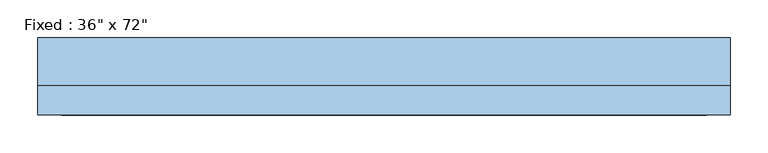
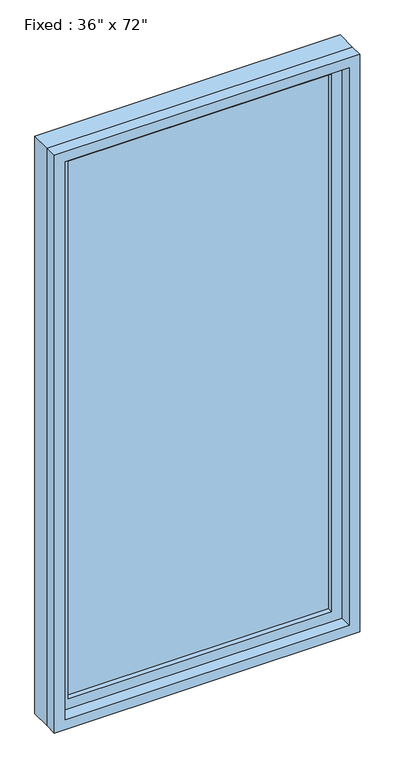
"""IFC4 building model written with IfcOpenShell, lengths in millimetres: window geometry."""

from ifc_helpers import new_model, si_unit, frame, origin, place, context, project, spatial, polyline, outline, extrude, source, transform, mapped, element, save


def window_8ce0b82f(model_context):
    return source(origin(), model_context, "Body", "SweptSolid", [
        extrude(outline(polyline([(355.6, 3.175), (-431.8, 3.175), (-431.8, 15.875), (355.6, 15.875), (355.6, 3.175)])), frame((0.0, 0.0, 368.3), z_axis=(0.0, 0.0, 1.0), x_axis=(1.0, 0.0, 0.0)), (0.0, 0.0, 1.0), 1701.8),
        extrude(outline(polyline([(2114.55, -476.25), (323.85, -476.25), (323.85, 400.05), (2114.55, 400.05), (2114.55, -476.25)]), holes=[polyline([(2070.1, -431.8), (2070.1, 355.6), (368.3, 355.6), (368.3, -431.8), (2070.1, -431.8)])]), frame((0.0, -12.7, 0.0), z_axis=(0.0, 1.0, 0.0), x_axis=(0.0, 0.0, 1.0)), (0.0, 0.0, 1.0), 44.45),
        extrude(outline(polyline([(2133.6, -495.3), (304.8, -495.3), (304.8, 419.1), (2133.6, 419.1), (2133.6, -495.3)]), holes=[polyline([(2101.85, -463.55), (2101.85, 387.35), (336.55, 387.35), (336.55, -463.55), (2101.85, -463.55)])]), frame((0.0, -50.8, 0.0), z_axis=(0.0, 1.0, 0.0), x_axis=(0.0, 0.0, 1.0)), (0.0, 0.0, 1.0), 38.1),
        extrude(outline(polyline([(2133.6, 419.1), (2133.6, -495.3), (304.8, -495.3), (304.8, 419.1), (2133.6, 419.1)]), holes=[polyline([(2114.55, 400.05), (323.85, 400.05), (323.85, -476.25), (2114.55, -476.25), (2114.55, 400.05)])]), frame((0.0, -12.7, 0.0), z_axis=(0.0, 1.0, 0.0), x_axis=(0.0, 0.0, 1.0)), (0.0, 0.0, 1.0), 63.5),
    ])


if __name__ == "__main__":
    model = new_model("IFC4")
    model_context = context("Model", 3, world=origin())
    ifc_project = project(units=[si_unit("LENGTHUNIT", "METRE", prefix="MILLI")], contexts=[model_context])
    site = spatial("IfcSite", under=ifc_project)
    building = spatial("IfcBuilding", under=site)
    placement = place(None, origin())
    window_shape = window_8ce0b82f(model_context)
    element("IfcWindow", 1, ObjectType="Fixed : 36\" x 72\"", at=placement, inside=building, context=model_context, shape_type="MappedRepresentation", body=[
        mapped(window_shape, transform((0.0, 0.0, 0.0), x_axis=(1.0, 0.0, 0.0), y_axis=(0.0, 1.0, 0.0), z_axis=(0.0, 0.0, 1.0))),
    ])
    save(model, "model.ifc")

# Revit data of these elements
# Type "Fixed : 36\" x 72\""
#   Type Mark = "9"
#   Construction Type Id = "GSP4R"
#   Assembly Code = "B2020100"
#   Analytic Construction = "1/8 in Pilkington single glazing"
#   Visual Light Transmittance = 0.9
#   Solar Heat Gain Coefficient = 0.78
#   Heat Transfer Coefficient (U) = 0.6496 BTU/(h·ft²·°F)
#   Height = 6' - 0"
#   Default Sill Height = 1' - 0"
#   Width = 3' - 0"
#   Window Inset = 0' - 0 3/4"
#   Define Thermal Properties by = 1
#   Glass Pane Material = Glass
#   Sash Material = Sash
#   Wall Closure = (empty or 0)
# Element 1 (IfcWindow, "Fixed : 36\" x 72\"")
#   Materials on its faces: "Sash", "Glass"
# Materials
#   "Glass": class "Glass", colour RGB 0 128 192, transparency 0.75, Description = "Soda Lime Glass", Cost = 0
#   "Sash": class "Wood", colour RGB 224 178 126, transparency 0
